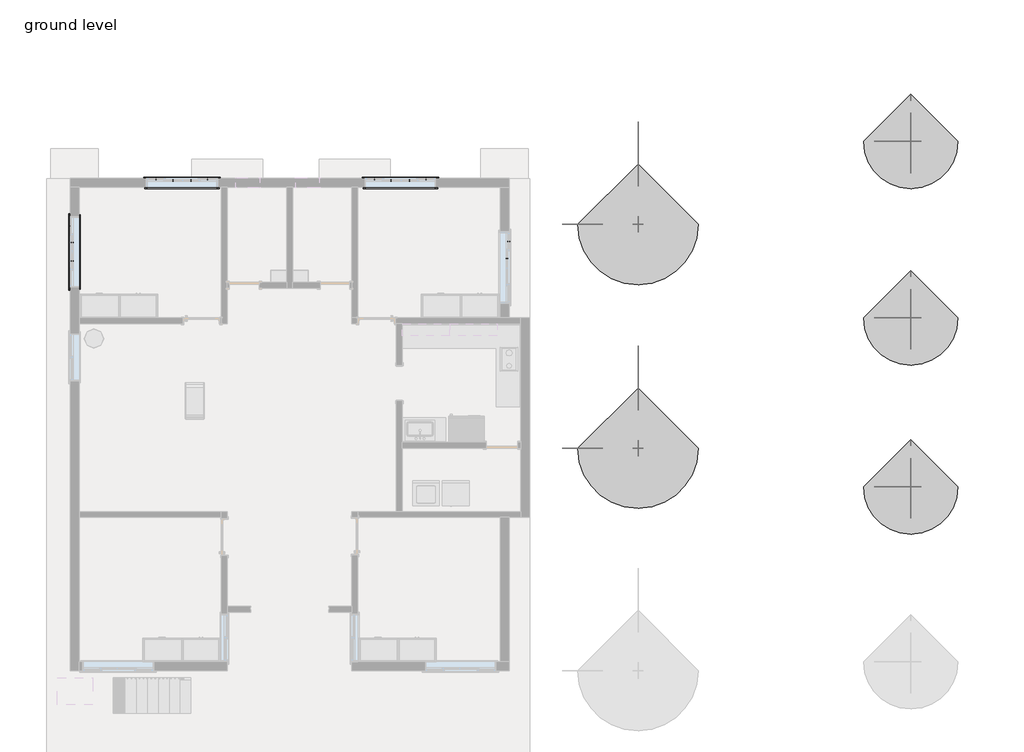
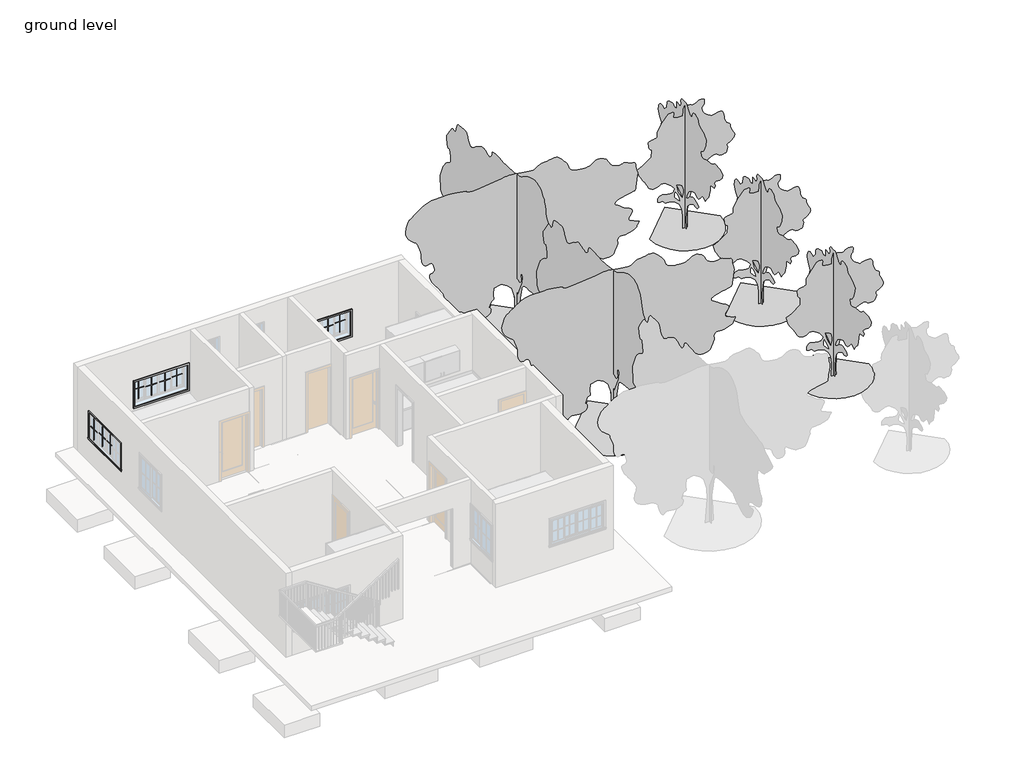
# One storey, part 4 of 4: 19 proxies, 5 geographic elements.
"""IFC4 building model written with IfcOpenShell, lengths in millimetres."""

from ifc_helpers import new_model, si_unit, origin, place, context, project, spatial, transform, mapped, element, save
from components import muntin_pattern_2x2_muntin_pattern_2x2_31a16349, trim_window_exterior_flat_with_sill_3c945769, trim_window_interior_flat_picture_frame_0edfbaa2, rpc_tree_deciduous_common_apple_20_2cf08d23, rpc_tree_deciduous_japanese_cherry_15_e499737d

model = new_model("IFC4")

# Units and contexts
model_context = context("Model", 3, world=origin())
ifc_project = project(units=[si_unit("LENGTHUNIT", "METRE", prefix="MILLI")], contexts=[model_context])

# Site, building, storey
site = spatial("IfcSite", under=ifc_project)
building = spatial("IfcBuilding", under=site)
storey = spatial("IfcBuildingStorey", under=building, Name="ground level", Elevation=609.6)

# Proxies
placement = place(None, origin())
muntin_pattern_2x2_muntin_pattern_2x2_shape = muntin_pattern_2x2_muntin_pattern_2x2_31a16349(model_context)
element("IfcBuildingElementProxy", 1, Name="Muntin Pattern_2x2 : Muntin Pattern_2x2", ObjectType="Muntin Pattern_2x2 : Muntin Pattern_2x2", at=placement, inside=storey, context=model_context, shape_type="MappedRepresentation", body=[
    mapped(muntin_pattern_2x2_muntin_pattern_2x2_shape, transform((-10432.4124084, 10171.2711804, 1606.55), x_axis=(1.0, 0.0, 0.0), y_axis=(0.0, 1.0, 0.0), z_axis=(0.0, 0.0, 1.0))),
])
element("IfcBuildingElementProxy", 2, Name="Muntin Pattern_2x2 : Muntin Pattern_2x2", ObjectType="Muntin Pattern_2x2 : Muntin Pattern_2x2", at=placement, inside=storey, context=model_context, shape_type="MappedRepresentation", body=[
    mapped(muntin_pattern_2x2_muntin_pattern_2x2_shape, transform((-10006.9624084, 10126.8211804, 1606.55), x_axis=(1.0, 0.0, 0.0), y_axis=(0.0, 1.0, 0.0), z_axis=(0.0, 0.0, 1.0))),
])
element("IfcBuildingElementProxy", 3, Name="Muntin Pattern_2x2 : Muntin Pattern_2x2", ObjectType="Muntin Pattern_2x2 : Muntin Pattern_2x2", at=placement, inside=storey, context=model_context, shape_type="MappedRepresentation", body=[
    mapped(muntin_pattern_2x2_muntin_pattern_2x2_shape, transform((-9537.0624084, 10126.8211804, 1606.55), x_axis=(1.0, 0.0, 0.0), y_axis=(0.0, 1.0, 0.0), z_axis=(0.0, 0.0, 1.0))),
])
element("IfcBuildingElementProxy", 4, Name="Muntin Pattern_2x2 : Muntin Pattern_2x2", ObjectType="Muntin Pattern_2x2 : Muntin Pattern_2x2", at=placement, inside=storey, context=model_context, shape_type="MappedRepresentation", body=[
    mapped(muntin_pattern_2x2_muntin_pattern_2x2_shape, transform((-9111.6124084, 10171.2711804, 1606.55), x_axis=(1.0, 0.0, 0.0), y_axis=(0.0, 1.0, 0.0), z_axis=(0.0, 0.0, 1.0))),
])
element("IfcBuildingElementProxy", 5, Name="Muntin Pattern_2x2 : Muntin Pattern_2x2", ObjectType="Muntin Pattern_2x2 : Muntin Pattern_2x2", at=placement, inside=storey, context=model_context, shape_type="MappedRepresentation", body=[
    mapped(muntin_pattern_2x2_muntin_pattern_2x2_shape, transform((-12588.2374084, 8059.8961804, 1606.55), x_axis=(0.0, 1.0, 0.0), y_axis=(-1.0, 0.0, 0.0), z_axis=(0.0, 0.0, 1.0))),
])
element("IfcBuildingElementProxy", 6, Name="Muntin Pattern_2x2 : Muntin Pattern_2x2", ObjectType="Muntin Pattern_2x2 : Muntin Pattern_2x2", at=placement, inside=storey, context=model_context, shape_type="MappedRepresentation", body=[
    mapped(muntin_pattern_2x2_muntin_pattern_2x2_shape, transform((-12588.2374084, 8529.7961804, 1606.55), x_axis=(0.0, 1.0, 0.0), y_axis=(-1.0, 0.0, 0.0), z_axis=(0.0, 0.0, 1.0))),
])
element("IfcBuildingElementProxy", 7, Name="Muntin Pattern_2x2 : Muntin Pattern_2x2", ObjectType="Muntin Pattern_2x2 : Muntin Pattern_2x2", at=placement, inside=storey, context=model_context, shape_type="MappedRepresentation", body=[
    mapped(muntin_pattern_2x2_muntin_pattern_2x2_shape, transform((-12632.6874084, 8955.2461804, 1606.55), x_axis=(0.0, 1.0, 0.0), y_axis=(-1.0, 0.0, 0.0), z_axis=(0.0, 0.0, 1.0))),
])
element("IfcBuildingElementProxy", 8, Name="Muntin Pattern_2x2 : Muntin Pattern_2x2", ObjectType="Muntin Pattern_2x2 : Muntin Pattern_2x2", at=placement, inside=storey, context=model_context, shape_type="MappedRepresentation", body=[
    mapped(muntin_pattern_2x2_muntin_pattern_2x2_shape, transform((-1374.1374084, 8555.1961804, 1606.55), x_axis=(0.0, -1.0, 0.0), y_axis=(1.0, 0.0, 0.0), z_axis=(0.0, 0.0, 1.0))),
])
element("IfcBuildingElementProxy", 9, Name="Muntin Pattern_2x2 : Muntin Pattern_2x2", ObjectType="Muntin Pattern_2x2 : Muntin Pattern_2x2", at=placement, inside=storey, context=model_context, shape_type="MappedRepresentation", body=[
    mapped(muntin_pattern_2x2_muntin_pattern_2x2_shape, transform((-1418.5874084, 8129.7461804, 1606.55), x_axis=(0.0, -1.0, 0.0), y_axis=(1.0, 0.0, 0.0), z_axis=(0.0, 0.0, 1.0))),
])
element("IfcBuildingElementProxy", 10, Name="Muntin Pattern_2x2 : Muntin Pattern_2x2", ObjectType="Muntin Pattern_2x2 : Muntin Pattern_2x2", at=placement, inside=storey, context=model_context, shape_type="MappedRepresentation", body=[
    mapped(muntin_pattern_2x2_muntin_pattern_2x2_shape, transform((-4819.0124084, 10171.2711804, 1606.55), x_axis=(1.0, 0.0, 0.0), y_axis=(0.0, 1.0, 0.0), z_axis=(0.0, 0.0, 1.0))),
])
element("IfcBuildingElementProxy", 11, Name="Muntin Pattern_2x2 : Muntin Pattern_2x2", ObjectType="Muntin Pattern_2x2 : Muntin Pattern_2x2", at=placement, inside=storey, context=model_context, shape_type="MappedRepresentation", body=[
    mapped(muntin_pattern_2x2_muntin_pattern_2x2_shape, transform((-4393.5624084, 10126.8211804, 1606.55), x_axis=(1.0, 0.0, 0.0), y_axis=(0.0, 1.0, 0.0), z_axis=(0.0, 0.0, 1.0))),
])
element("IfcBuildingElementProxy", 12, Name="Muntin Pattern_2x2 : Muntin Pattern_2x2", ObjectType="Muntin Pattern_2x2 : Muntin Pattern_2x2", at=placement, inside=storey, context=model_context, shape_type="MappedRepresentation", body=[
    mapped(muntin_pattern_2x2_muntin_pattern_2x2_shape, transform((-3923.6624084, 10126.8211804, 1606.55), x_axis=(1.0, 0.0, 0.0), y_axis=(0.0, 1.0, 0.0), z_axis=(0.0, 0.0, 1.0))),
])
element("IfcBuildingElementProxy", 13, Name="Muntin Pattern_2x2 : Muntin Pattern_2x2", ObjectType="Muntin Pattern_2x2 : Muntin Pattern_2x2", at=placement, inside=storey, context=model_context, shape_type="MappedRepresentation", body=[
    mapped(muntin_pattern_2x2_muntin_pattern_2x2_shape, transform((-3498.2124084, 10171.2711804, 1606.55), x_axis=(1.0, 0.0, 0.0), y_axis=(0.0, 1.0, 0.0), z_axis=(0.0, 0.0, 1.0))),
])
trim_window_exterior_flat_with_sill_shape = trim_window_exterior_flat_with_sill_3c945769(model_context)
element("IfcBuildingElementProxy", 14, Name="Trim-Window-Exterior-Flat : with Sill", ObjectType="Trim-Window-Exterior-Flat : with Sill", at=placement, inside=storey, context=model_context, shape_type="MappedRepresentation", body=[
    mapped(trim_window_exterior_flat_with_sill_shape, transform((-9772.0124084, 10180.7961804, 2438.4), x_axis=(-1.0, 0.0, 0.0), y_axis=(0.0, 0.0, 1.0), z_axis=(0.0, 1.0, 0.0))),
])
element("IfcBuildingElementProxy", 15, Name="Trim-Window-Exterior-Flat : with Sill", ObjectType="Trim-Window-Exterior-Flat : with Sill", at=placement, inside=storey, context=model_context, shape_type="MappedRepresentation", body=[
    mapped(trim_window_exterior_flat_with_sill_shape, transform((-12642.2124084, 8294.8461804, 2438.4), x_axis=(0.0, -1.0, 0.0), y_axis=(0.0, 0.0, 1.0), z_axis=(-1.0, 0.0, 0.0))),
])
element("IfcBuildingElementProxy", 16, Name="Trim-Window-Exterior-Flat : with Sill", ObjectType="Trim-Window-Exterior-Flat : with Sill", at=placement, inside=storey, context=model_context, shape_type="MappedRepresentation", body=[
    mapped(trim_window_exterior_flat_with_sill_shape, transform((-4158.6124084, 10180.7961804, 2438.4), x_axis=(-1.0, 0.0, 0.0), y_axis=(0.0, 0.0, 1.0), z_axis=(0.0, 1.0, 0.0))),
])
trim_window_interior_flat_picture_frame_shape = trim_window_interior_flat_picture_frame_0edfbaa2(model_context)
element("IfcBuildingElementProxy", 17, Name="Trim-Window-Interior-Flat : Picture Frame", ObjectType="Trim-Window-Interior-Flat : Picture Frame", at=placement, inside=storey, context=model_context, shape_type="MappedRepresentation", body=[
    mapped(trim_window_interior_flat_picture_frame_shape, transform((-9772.0124084, 9952.1961804, 2438.4), x_axis=(1.0, 0.0, 0.0), y_axis=(0.0, 0.0, 1.0), z_axis=(0.0, -1.0, 0.0))),
])
element("IfcBuildingElementProxy", 18, Name="Trim-Window-Interior-Flat : Picture Frame", ObjectType="Trim-Window-Interior-Flat : Picture Frame", at=placement, inside=storey, context=model_context, shape_type="MappedRepresentation", body=[
    mapped(trim_window_interior_flat_picture_frame_shape, transform((-12413.6124084, 8294.8461804, 2438.4), x_axis=(0.0, 1.0, 0.0), y_axis=(0.0, 0.0, 1.0), z_axis=(1.0, 0.0, 0.0))),
])
element("IfcBuildingElementProxy", 19, Name="Trim-Window-Interior-Flat : Picture Frame", ObjectType="Trim-Window-Interior-Flat : Picture Frame", at=placement, inside=storey, context=model_context, shape_type="MappedRepresentation", body=[
    mapped(trim_window_interior_flat_picture_frame_shape, transform((-4158.6124084, 9952.1961804, 2438.4), x_axis=(1.0, 0.0, 0.0), y_axis=(0.0, 0.0, 1.0), z_axis=(0.0, -1.0, 0.0))),
])

# Geographic elements
rpc_tree_deciduous_common_apple_20_shape = rpc_tree_deciduous_common_apple_20_2cf08d23(model_context)
element("IfcGeographicElement", 20, ObjectType="RPC Tree - Deciduous : Common Apple - 20'", at=placement, inside=storey, context=model_context, shape_type="MappedRepresentation", body=[
    mapped(rpc_tree_deciduous_common_apple_20_shape, transform((1950.0875916, 8999.6961804, 457.2), x_axis=(1.0, 0.0, 0.0), y_axis=(0.0, 1.0, 0.0), z_axis=(0.0, 0.0, 1.0))),
])
element("IfcGeographicElement", 21, ObjectType="RPC Tree - Deciduous : Common Apple - 20'", at=placement, inside=storey, context=model_context, shape_type="MappedRepresentation", body=[
    mapped(rpc_tree_deciduous_common_apple_20_shape, transform((1950.0875916, 3246.5961804, 457.2), x_axis=(1.0, 0.0, 0.0), y_axis=(0.0, 1.0, 0.0), z_axis=(0.0, 0.0, 1.0))),
])
rpc_tree_deciduous_japanese_cherry_15_shape = rpc_tree_deciduous_japanese_cherry_15_e499737d(model_context)
element("IfcGeographicElement", 22, ObjectType="RPC Tree - Deciduous : Japanese Cherry - 15'", at=placement, inside=storey, context=model_context, shape_type="MappedRepresentation", body=[
    mapped(rpc_tree_deciduous_japanese_cherry_15_shape, transform((8960.4875916, 11133.2961804, 457.2), x_axis=(1.0, 0.0, 0.0), y_axis=(0.0, 1.0, 0.0), z_axis=(0.0, 0.0, 1.0))),
])
element("IfcGeographicElement", 23, ObjectType="RPC Tree - Deciduous : Japanese Cherry - 15'", at=placement, inside=storey, context=model_context, shape_type="MappedRepresentation", body=[
    mapped(rpc_tree_deciduous_japanese_cherry_15_shape, transform((8960.4875916, 6599.3961804, 457.2), x_axis=(1.0, 0.0, 0.0), y_axis=(0.0, 1.0, 0.0), z_axis=(0.0, 0.0, 1.0))),
])
element("IfcGeographicElement", 24, ObjectType="RPC Tree - Deciduous : Japanese Cherry - 15'", at=placement, inside=storey, context=model_context, shape_type="MappedRepresentation", body=[
    mapped(rpc_tree_deciduous_japanese_cherry_15_shape, transform((8960.4875916, 2255.9961804, 457.2), x_axis=(1.0, 0.0, 0.0), y_axis=(0.0, 1.0, 0.0), z_axis=(0.0, 0.0, 1.0))),
])

save(model, "model.ifc")

# Revit data of these elements
# Type "Muntin Pattern_2x2 : Muntin Pattern_2x2"
#   Width [instance default] = 4' - 0"
#   Thickness = 0' - 0 1/2"
#   Height [instance default] = 4' - 0"
#   Distance = 0' - 0 3/4"
#   Interior Material [instance default] = none
#   Exterior Material [instance default] = none
#   Default Elevation = 0
# Type "Trim-Window-Exterior-Flat : with Sill"
#   Trim Width = 0' - 2 1/4"
#   Trim Thickness_Picture Frame = 0' - 1 1/4"
#   Trim Thickness_with Sill = 0' - 0 3/4"
#   Sill Thickness = 0' - 1 1/4"
#   Opening Width [instance default] = 2' - 0"
#   Opening Height [instance default] = 3' - 0"
#   Default Elevation = 4' - 0"
#   Sill = yes
#   Picture Frame = no
#   Trim Material [instance default] = none
# Type "Trim-Window-Interior-Flat : Picture Frame"
#   Trim Thickness_Picture Frame = 0' - 1 1/4"
#   Trim Width = 0' - 2 1/4"
#   Trim Thickness_with Sill = 0' - 0 3/4"
#   Sill Thickness = 0' - 1 1/4"
#   Opening Width [instance default] = 2' - 0"
#   Opening Height [instance default] = 3' - 0"
#   Default Elevation = 4' - 0"
#   Sill = no
#   Picture Frame = yes
#   Trim Material [instance default] = none
# Type "RPC Tree - Deciduous : Common Apple - 20'"
#   built-in parameter 1005198 = "{2, 15},{39, RPC-16-FXGK-4KXX-PJE5-6000-ST1L-LVER-AU},{1, 0},{1, 0},{2, 35},{1, 8},{5, Color},{1, 0},{1, 0},{3, 0.8},{3, 0.8},{3, 0.8},{1, 8},{7, BBoxMin},{1, 0},{1, 0},{1, 0},{1, 0},{1, 0},{1, 8},{7, BBoxMax},{1, 0},{1, 0},{1, 0},{1, 0},{1, 0},{2, 11},{9, RPCTypeId},{1, 0},{1, 0},{39, RPC-16-FXGK-4KXX-PJE5-6000-ST1L-LVER-AU},{1, 6},{14, RPCPlantHeight},{1, 0},{1, 0},{2, 20},{2, 11},{7, keyword},{1, 0},{1, 0},{168, :Geometry:RPC:Common Apple:Malus sylvestris:occurs in southern Ontario near Lakes Erie and Ontario.  Numerous cultivars planted in orchards; naturalized in many places.},{2, 11},{8, category},{1, 0},{1, 0},{16, :Trees [General]},{2, 11},{12, LocalizedUID},{1, 0},{1, 0},{12, Common Apple},{2, 14},{6, Height},{1, 0},{1, 0},{2, 20},{1, 2},{16, Cast Reflections},{1, 0},{1, 0},{1, 0},{1, 2},{12, Cast Shadows},{1, 0},{1, 0},{1, 1},{1, 2},{9, Lock View},{1, 0},{1, 0},{1, 0},{1, 4},{5, ViewC},{1, 0},{1, 0},{1, 0},{2, 11},{20, AdvancedUIDefinition},{1, 0},{1, 0},{0, },{2, 11},{10, AssetLibID},{1, 0},{1, 0},{36, 4D3F6E72-3F99-4203-98E9-AF80B3C7A7A4},{2, 11},{10, BaseSchema},{1, 0},{1, 0},{9, RPCSchema},{2, 11},{12, ExchangeGUID},{1, 0},{1, 0},{0, },{1, 2},{6, Hidden},{1, 0},{1, 0},{1, 0},{1, 4},{11, RPCCategory},{1, 0},{1, 0},{1, 0},{2, 11},{8, RPCImage},{1, 0},{1, 0},{0, },{1, 4},{13, SchemaVersion},{1, 0},{1, 0},{1, 4},{2, 11},{12, UIDefinition},{1, 0},{1, 0},{0, },{2, 11},{6, UIName},{1, 0},{1, 0},{39, RPC-16-FXGK-4KXX-PJE5-6000-ST1L-LVER-AU},{2, 11},{11, VersionGUID},{1, 0},{1, 0},{9, RPCSchema},{2, 11},{9, assettype},{1, 0},{1, 0},{11, RPCGeometry},{2, 11},{11, description},{1, 0},{1, 0},{0, },{2, 11},{9, localname},{1, 0},{1, 0},{3, RPC},{2, 11},{9, localtype},{1, 0},{1, 0},{3, RPC},{1, 4},{8, revision},{1, 0},{1, 0},{1, 1},{2, 11},{9, thumbnail},{1, 0},{1, 0},{0, },{1, 4},{7, version},{1, 0},{1, 0},{1, 1},{1, 2},{20, RPC_Cast Reflections},{1, 0},{1, 0},{1, 1},{1, 2},{16, RPC_Cast Shadows},{1, 0},{1, 0},{1, 1},{1, 2},{13, RPC_Lock View},{1, 0},{1, 0},{1, 0},{1, 4},{9, RPC_ViewC},{1, 0},{1, 0},{1, 0},{21, assetlibrary_base.fbx},{1, 5},"
#   built-in parameter 1005195 = "RPC-16-FXGK-4KXX-PJE5-6000-ST1L-LVER-AU"
#   Type Comments = "Common Apple"
#   Assembly Code = "G2050500"
#   Height = 20' - 0"
#   Default Elevation = 0
# Type "RPC Tree - Deciduous : Japanese Cherry - 15'"
#   built-in parameter 1005198 = "{2, 15},{39, RPC-16-FXGW-2MQ0-PN7K-A000-ST1L-LVER-AU},{1, 0},{1, 0},{2, 35},{1, 8},{5, Color},{1, 0},{1, 0},{3, 0.8},{3, 0.8},{3, 0.8},{1, 8},{7, BBoxMin},{1, 0},{1, 0},{1, 0},{1, 0},{1, 0},{1, 8},{7, BBoxMax},{1, 0},{1, 0},{1, 0},{1, 0},{1, 0},{2, 11},{9, RPCTypeId},{1, 0},{1, 0},{39, RPC-16-FXGW-2MQ0-PN7K-A000-ST1L-LVER-AU},{1, 6},{14, RPCPlantHeight},{1, 0},{1, 0},{2, 15},{2, 11},{7, keyword},{1, 0},{1, 0},{207, :Geometry:RPC:Japanese Flowering Cherry:Prunus serrulata Lindl:A landscape tree:valued for its abundant showy flowers; native to China and Japan.  Hardy only in the mildest parts of Canada and farther south.},{2, 11},{8, category},{1, 0},{1, 0},{16, :Trees [General]},{2, 11},{12, LocalizedUID},{1, 0},{1, 0},{25, Japanese Flowering Cherry},{2, 14},{6, Height},{1, 0},{1, 0},{2, 15},{1, 2},{16, Cast Reflections},{1, 0},{1, 0},{1, 0},{1, 2},{12, Cast Shadows},{1, 0},{1, 0},{1, 1},{1, 2},{9, Lock View},{1, 0},{1, 0},{1, 0},{1, 4},{5, ViewC},{1, 0},{1, 0},{1, 0},{2, 11},{20, AdvancedUIDefinition},{1, 0},{1, 0},{0, },{2, 11},{10, AssetLibID},{1, 0},{1, 0},{36, 4D3F6E72-3F99-4203-98E9-AF80B3C7A7A4},{2, 11},{10, BaseSchema},{1, 0},{1, 0},{9, RPCSchema},{2, 11},{12, ExchangeGUID},{1, 0},{1, 0},{0, },{1, 2},{6, Hidden},{1, 0},{1, 0},{1, 0},{1, 4},{11, RPCCategory},{1, 0},{1, 0},{1, 0},{2, 11},{8, RPCImage},{1, 0},{1, 0},{0, },{1, 4},{13, SchemaVersion},{1, 0},{1, 0},{1, 4},{2, 11},{12, UIDefinition},{1, 0},{1, 0},{0, },{2, 11},{6, UIName},{1, 0},{1, 0},{39, RPC-16-FXGW-2MQ0-PN7K-A000-ST1L-LVER-AU},{2, 11},{11, VersionGUID},{1, 0},{1, 0},{9, RPCSchema},{2, 11},{9, assettype},{1, 0},{1, 0},{11, RPCGeometry},{2, 11},{11, description},{1, 0},{1, 0},{0, },{2, 11},{9, localname},{1, 0},{1, 0},{3, RPC},{2, 11},{9, localtype},{1, 0},{1, 0},{3, RPC},{1, 4},{8, revision},{1, 0},{1, 0},{1, 1},{2, 11},{9, thumbnail},{1, 0},{1, 0},{0, },{1, 4},{7, version},{1, 0},{1, 0},{1, 1},{1, 2},{20, RPC_Cast Reflections},{1, 0},{1, 0},{1, 1},{1, 2},{16, RPC_Cast Shadows},{1, 0},{1, 0},{1, 1},{1, 2},{13, RPC_Lock View},{1, 0},{1, 0},{1, 0},{1, 4},{9, RPC_ViewC},{1, 0},{1, 0},{1, 0},{21, assetlibrary_base.fbx},{1, 5},"
#   built-in parameter 1005195 = "RPC-16-FXGW-2MQ0-PN7K-A000-ST1L-LVER-AU"
#   Type Comments = "Japanese Cherry"
#   Assembly Code = "G2050500"
#   Height = 15' - 0"
#   Default Elevation = 0
# Elements 1, 2, 3, 4, 5, 6, 7, 8, 9, 10, 11, 12, 13 (IfcBuildingElementProxy, "Muntin Pattern_2x2 : Muntin Pattern_2x2")
#   Width = 1' - 3"
#   Height = 2' - 6 1/4"
#   Interior Material = Wood - Stained
#   Exterior Material = Clad - White
#   Phase Created = New Construction
#   Materials on its faces: "Clad - White", "Wood - Stained"
# Elements 14, 15, 16 (IfcBuildingElementProxy, "Trim-Window-Exterior-Flat : with Sill")
#   Opening Width = 6' - 0"
#   Opening Height = 3' - 0"
#   Trim Material = Clad - White
#   Phase Created = New Construction
#   Materials on its faces: "Clad - White"
# Elements 17, 18, 19 (IfcBuildingElementProxy, "Trim-Window-Interior-Flat : Picture Frame")
#   Opening Width = 6' - 0"
#   Opening Height = 3' - 0"
#   Trim Material = Wood - Stained
#   Phase Created = New Construction
#   Materials on its faces: "Wood - Stained"
# Elements 20, 21 (IfcGeographicElement, "RPC Tree - Deciduous : Common Apple - 20'")
#   Phase Created = New Construction
# Elements 22, 23, 24 (IfcGeographicElement, "RPC Tree - Deciduous : Japanese Cherry - 15'")
#   Phase Created = New Construction
# Materials
#   "Clad - White": class "Wood", colour RGB 242 242 238, transparency 0, Cost = 0
#   "Wood - Stained": class "Wood", colour RGB 224 178 126, transparency 0, Cost = 0
